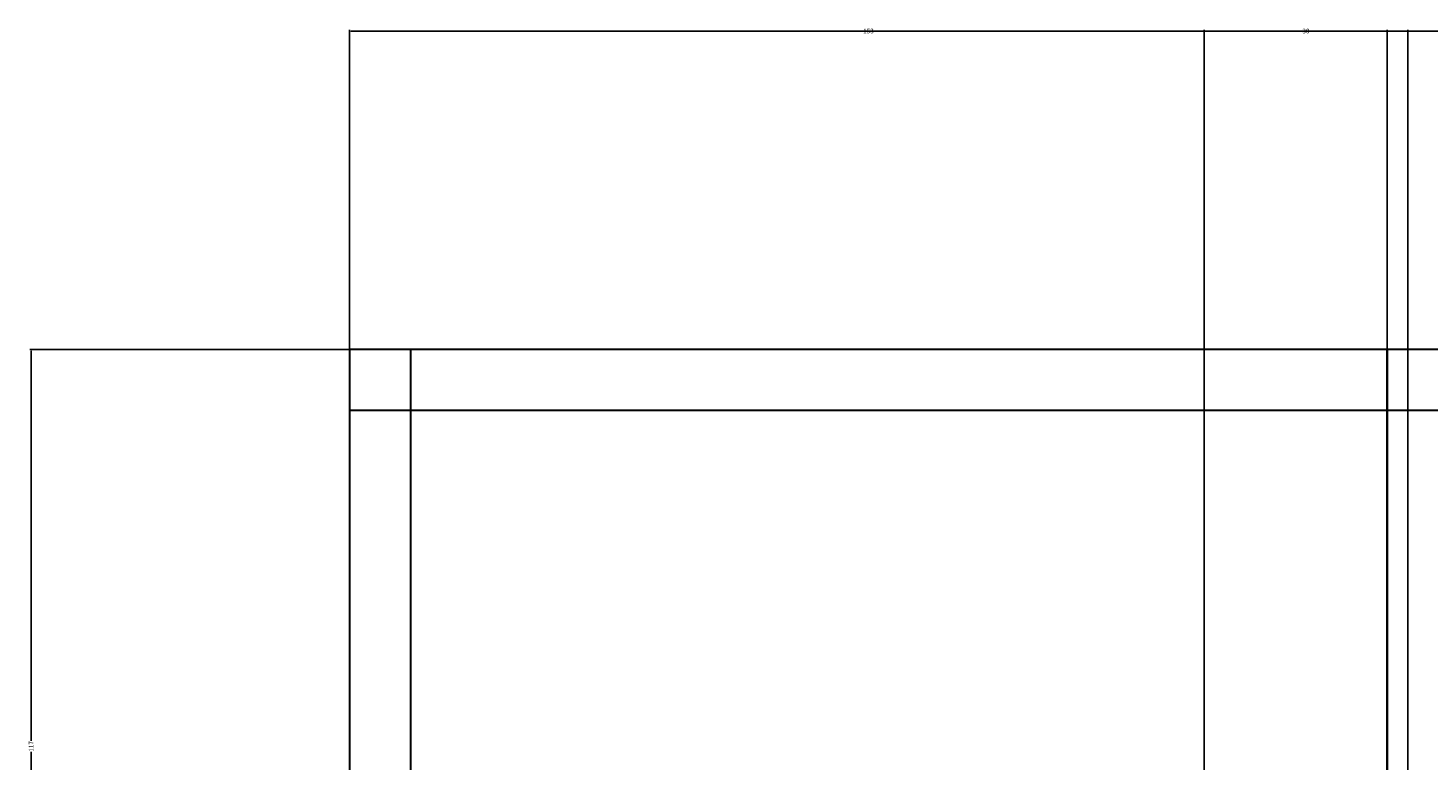
# Model space of a CAD drawing. Units: inches. Extents: x 867 to 1667, y -234 to 788.
# Tile 31 of 42: x 867 to 1074, y 680 to 788. Entities that reach past the tile are written whole.
import ezdxf

# ---------------------------------------------------------------- set-up
doc = ezdxf.new("R2010")
doc.units = ezdxf.units.IN
doc.header["$MEASUREMENT"] = 0
for name, color, linetype, lineweight in [('A-ANNO-DIMS', 2, 'Continuous', 18), ('A-Wall', 7, 'Continuous', 35), ('A-WALL-SITE', 8, 'Continuous', 30)]:
    doc.layers.add(name, color=color, linetype=linetype, lineweight=lineweight)
doc.styles.get("Standard").update_dxf_attribs({"font": 'arial.ttf'})
doc.dimstyles.get("Standard").update_dxf_attribs({"dimtxt": 0.6875, "dimasz": 0.18, "dimexe": 0.18, "dimexo": 0.0625, "dimgap": 0.09, "dimtad": 0, "dimdec": 4, "dimzin": 0, "dimdsep": 46, "dimlunit": 4, "dimtxsty": 'Standard', "dimcen": 0.09, "dimadec": 0, "dimazin": 0, "dimtfac": 1, "dimtdec": 4, "dimtofl": 0, "dimtmove": 0, "dimatfit": 3, "dimfxl": 1, "dimtolj": 1, "dimtzin": 0, "dimarcsym": 0})

# ---------------------------------------------------------------- blocks, each defined once
blk = doc.blocks.new('*D17')
at = {"layer": 'A-ANNO-DIMS', "color": 0, "lineweight": -2, "transparency": 16777216}
for p, q in [((914.89, 740.68), (914.89, 787.75)), ((915.07, 787.57), (1266.54, 787.57)), ((1619.71, 787.57), (1268.24, 787.57)), ((1619.89, 740.68), (1619.89, 787.75))]:
    blk.add_line(p, q, dxfattribs=at)
at = {"layer": 'A-ANNO-DIMS', "color": 0, "transparency": 16777216}
for points in [[(915.07, 787.6), (915.07, 787.54), (914.89, 787.57)], [(1619.71, 787.6), (1619.71, 787.54), (1619.89, 787.57)]]:
    blk.add_solid(points, dxfattribs=at)
at = {"layer": 'Defpoints', "color": 0, "transparency": 16777216}
for p in [(1619.89, 787.57), (914.89, 740.62), (1619.89, 740.62)]:
    blk.add_point(p, dxfattribs=at)
at = {"layer": 'A-ANNO-DIMS', "color": 0, "transparency": 16777216, "insert": (1267.39, 787.57), "char_height": 0.688, "attachment_point": 5}
blk.add_mtext('\\A1;705', dxfattribs=at)
blk = doc.blocks.new('*D19')
at = {"layer": 'A-ANNO-DIMS', "color": 0, "lineweight": -2, "transparency": 16777216}
for p, q in [((914.82, 740.62), (867.76, 740.62)), ((867.94, 740.44), (867.94, 682.93)), ((867.94, 623.8), (867.94, 681.3)), ((914.82, 623.62), (867.76, 623.62))]:
    blk.add_line(p, q, dxfattribs=at)
at = {"layer": 'A-ANNO-DIMS', "color": 0, "transparency": 16777216}
for points in [[(867.91, 740.44), (867.97, 740.44), (867.94, 740.62)], [(867.91, 623.8), (867.97, 623.8), (867.94, 623.62)]]:
    blk.add_solid(points, dxfattribs=at)
at = {"layer": 'Defpoints', "color": 0, "transparency": 16777216}
for p in [(867.94, 740.62), (914.89, 740.62), (914.89, 623.62)]:
    blk.add_point(p, dxfattribs=at)
at = {"layer": 'A-ANNO-DIMS', "color": 0, "transparency": 16777216, "insert": (867.94, 682.12), "char_height": 0.688, "attachment_point": 5, "rotation": 90}
blk.add_mtext('\\A1;117', dxfattribs=at)
blk = doc.blocks.new('*D20')
at = {"layer": 'A-ANNO-DIMS', "color": 0, "lineweight": -2, "transparency": 16777216}
for p, q in [((914.89, 740.68), (914.89, 787.75)), ((915.07, 787.57), (990.57, 787.57)), ((1067.71, 787.57), (992.2, 787.57)), ((1067.89, 740.68), (1067.89, 787.75))]:
    blk.add_line(p, q, dxfattribs=at)
at = {"layer": 'A-ANNO-DIMS', "color": 0, "transparency": 16777216}
for points in [[(915.07, 787.6), (915.07, 787.54), (914.89, 787.57)], [(1067.71, 787.6), (1067.71, 787.54), (1067.89, 787.57)]]:
    blk.add_solid(points, dxfattribs=at)
at = {"layer": 'Defpoints', "color": 0, "transparency": 16777216}
for p in [(1067.89, 787.57), (914.89, 740.62), (1067.89, 740.62)]:
    blk.add_point(p, dxfattribs=at)
at = {"layer": 'A-ANNO-DIMS', "color": 0, "transparency": 16777216, "insert": (991.39, 787.57), "char_height": 0.688, "attachment_point": 5}
blk.add_mtext('\\A1;153', dxfattribs=at)
blk = doc.blocks.new('*D21')
at = {"layer": 'A-ANNO-DIMS', "color": 0, "lineweight": -2, "transparency": 16777216}
for p, q in [((1067.89, 740.68), (1067.89, 787.75)), ((1068.07, 787.57), (1143.57, 787.57)), ((1220.71, 787.57), (1145.2, 787.57)), ((1220.89, 740.68), (1220.89, 787.75))]:
    blk.add_line(p, q, dxfattribs=at)
at = {"layer": 'A-ANNO-DIMS', "color": 0, "transparency": 16777216}
for points in [[(1068.07, 787.6), (1068.07, 787.54), (1067.89, 787.57)], [(1220.71, 787.6), (1220.71, 787.54), (1220.89, 787.57)]]:
    blk.add_solid(points, dxfattribs=at)
at = {"layer": 'Defpoints', "color": 0, "transparency": 16777216}
for p in [(1220.89, 787.57), (1067.89, 740.62), (1220.89, 740.62)]:
    blk.add_point(p, dxfattribs=at)
at = {"layer": 'A-ANNO-DIMS', "color": 0, "transparency": 16777216, "insert": (1144.39, 787.57), "char_height": 0.688, "attachment_point": 5}
blk.add_mtext('\\A1;153', dxfattribs=at)
blk = doc.blocks.new('*D31')
at = {"layer": 'A-ANNO-DIMS', "color": 0, "lineweight": -2, "transparency": 16777216}
for p, q in [((1070.89, 566.68), (1070.89, 787.75)), ((1071.07, 787.57), (1304.02, 787.57)), ((1538.71, 787.57), (1305.75, 787.57)), ((1538.89, 566.68), (1538.89, 787.75))]:
    blk.add_line(p, q, dxfattribs=at)
at = {"layer": 'A-ANNO-DIMS', "color": 0, "transparency": 16777216}
for points in [[(1071.07, 787.6), (1071.07, 787.54), (1070.89, 787.57)], [(1538.71, 787.6), (1538.71, 787.54), (1538.89, 787.57)]]:
    blk.add_solid(points, dxfattribs=at)
at = {"layer": 'Defpoints', "color": 0, "transparency": 16777216}
for p in [(1538.89, 787.57), (1070.89, 566.62), (1538.89, 566.62)]:
    blk.add_point(p, dxfattribs=at)
at = {"layer": 'A-ANNO-DIMS', "color": 0, "transparency": 16777216, "insert": (1304.89, 787.57), "char_height": 0.688, "attachment_point": 5}
blk.add_mtext('\\A1;468', dxfattribs=at)
blk = doc.blocks.new('*D35')
at = {"layer": 'A-ANNO-DIMS', "color": 0, "lineweight": -2, "transparency": 16777216}
for p, q in [((1040.89, 413.68), (1040.89, 787.75)), ((1041.07, 787.57), (1055.31, 787.57)), ((1070.71, 787.57), (1056.47, 787.57)), ((1070.89, 404.68), (1070.89, 787.75))]:
    blk.add_line(p, q, dxfattribs=at)
at = {"layer": 'A-ANNO-DIMS', "color": 0, "transparency": 16777216}
for points in [[(1041.07, 787.6), (1041.07, 787.54), (1040.89, 787.57)], [(1070.71, 787.6), (1070.71, 787.54), (1070.89, 787.57)]]:
    blk.add_solid(points, dxfattribs=at)
at = {"layer": 'Defpoints', "color": 0, "transparency": 16777216}
for p in [(1070.89, 787.57), (1040.89, 413.62), (1070.89, 404.62)]:
    blk.add_point(p, dxfattribs=at)
at = {"layer": 'A-ANNO-DIMS', "color": 0, "transparency": 16777216, "insert": (1055.89, 787.57), "char_height": 0.688, "attachment_point": 5}
blk.add_mtext('\\A1;30', dxfattribs=at)

msp = doc.modelspace()

# ---------------------------------------------------------------- linework, layer by layer
at = {"layer": 'A-Wall'}
msp.add_line((1067.8866, 740.617), (1067.8866, 623.617), dxfattribs=at)
at = {"layer": 'A-WALL-SITE'}
for p, q in [((914.8866, 740.617), (914.8866, -186.4081)), ((1619.8866, 740.617), (914.8866, 740.617)), ((923.8866, 740.617), (923.8866, -186.4081)), ((1619.8866, 731.617), (914.8866, 731.617))]:
    msp.add_line(p, q, dxfattribs=at)

# ---------------------------------------------------------------- dimensions: what is measured, and where the dimension line sits
at = {"layer": 'A-ANNO-DIMS'}
for base, p1, p2, picture, middle in [((1619.8866, 787.567), (914.8866, 740.617), (1619.8866, 740.617), '*D17', (1267.3866, 787.567)), ((1067.8866, 787.567), (914.8866, 740.617), (1067.8866, 740.617), '*D20', (991.3866, 787.567)), ((1070.8866, 787.567), (1040.8866, 413.617), (1070.8866, 404.617), '*D35', (1055.8866, 787.567)), ((1220.8866, 787.567), (1067.8866, 740.617), (1220.8866, 740.617), '*D21', (1144.3866, 787.567)), ((1538.8866, 787.567), (1070.8866, 566.617), (1538.8866, 566.617), '*D31', (1304.8866, 787.567))]:
    dim = msp.add_linear_dim(base=base, p1=p1, p2=p2, dimstyle='Standard', override={"dimdec": 0, "dimlfac": 1, "dimrnd": 0, "dimzin": 0, "dimdsep": 46, "dimlunit": 2}, dxfattribs=at)
    dim.commit()
    dim.dimension.update_dxf_attribs({"geometry": picture, "text_midpoint": middle})
dim = msp.add_linear_dim(base=(867.9366, 740.617), p1=(914.8866, 623.617), p2=(914.8866, 740.617), angle=90, dimstyle='Standard', override={"dimdec": 0, "dimlfac": 1, "dimrnd": 0, "dimzin": 0, "dimdsep": 46, "dimlunit": 2}, dxfattribs=at)
dim.commit()
dim.dimension.update_dxf_attribs({"geometry": '*D19', "text_midpoint": (867.9366, 682.117)})

doc.saveas('drawing.dxf')
